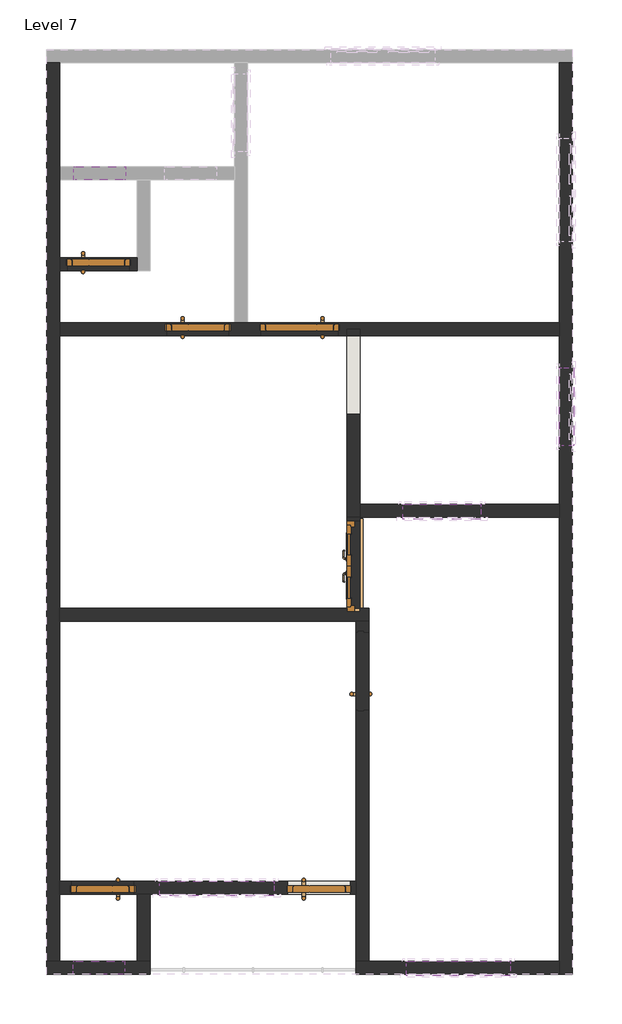
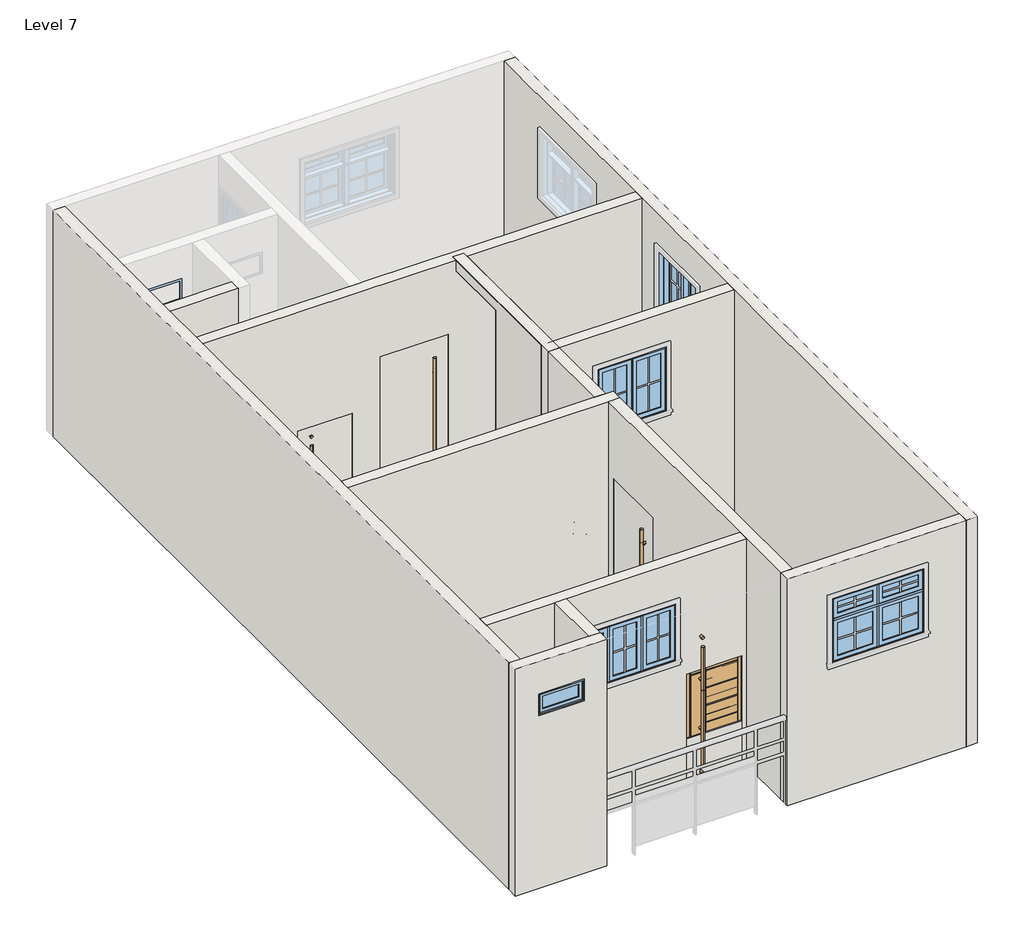
# One storey, part 1 of 2: 22 walls, 8 doors, 8 windows.
"""IFC4 building model written with IfcOpenShell, lengths in millimetres."""

from ifc_helpers import new_model, si_unit, frame, origin, place, context, project, spatial, polyline, outline, extrude, faceted_brep, transform, mapped, element, save
from components import door_9b787682, door_dc81b0c5, door_3_5c4206ef, door_3_79df91aa, door_2576ec39, door_55c03dfd, fixed_2_65c13adb, window_61697a4f, m_window_casement_double_3_e0bd8fa3, m_window_casement_double_awning_double_4_7efa9bbd

model = new_model("IFC4")

# Units and contexts
model_context = context("Model", 3, world=origin())
ifc_project = project(units=[si_unit("LENGTHUNIT", "METRE", prefix="MILLI")], contexts=[model_context])

# Site, building, storey
site = spatial("IfcSite", under=ifc_project)
building = spatial("IfcBuilding", under=site)
storey = spatial("IfcBuildingStorey", under=building, Name="Level 7", Elevation=10210.8)

# Doors
placement = place(None, origin())
door_shape = door_9b787682(model_context)
element("IfcDoor", 1, ObjectType="2'5\"", at=placement, inside=storey, context=model_context, shape_type="MappedRepresentation", body=[
    mapped(door_shape, transform((-22033.2963079, 3049.4742053, 10210.8), x_axis=(1.0, 0.0, 0.0), y_axis=(0.0, 1.0, 0.0), z_axis=(0.0, 0.0, 1.0))),
])
element("IfcDoor", 2, ObjectType="2'5\"", at=placement, inside=storey, context=model_context, shape_type="MappedRepresentation", body=[
    mapped(door_shape, transform((-23201.6963079, 3811.4742053, 10210.8), x_axis=(1.0, 0.0, 0.0), y_axis=(0.0, 1.0, 0.0), z_axis=(0.0, 0.0, 1.0))),
])
element("IfcDoor", 3, ObjectType="2'5\"", at=placement, inside=storey, context=model_context, shape_type="MappedRepresentation", body=[
    mapped(door_shape, transform((-23150.8963079, -3503.7257947, 10210.8), x_axis=(-1.0, 0.0, 0.0), y_axis=(0.0, -1.0, 0.0), z_axis=(0.0, 0.0, 1.0))),
])
door_2_shape = door_dc81b0c5(model_context)
element("IfcDoor", 4, ObjectType="2'5\"", at=placement, inside=storey, context=model_context, shape_type="MappedRepresentation", body=[
    mapped(door_2_shape, transform((-20610.8963079, -3503.7257947, 10257.0445349), x_axis=(1.0, 0.0, 0.0), y_axis=(0.0, 1.0, 0.0), z_axis=(0.0, 0.0, 1.0))),
])
element("IfcDoor", 5, ObjectType="2'5\"", at=placement, inside=storey, context=model_context, shape_type="MappedRepresentation", body=[
    mapped(door_2_shape, transform((-20610.8963079, -3503.7257947, 10866.6445349), x_axis=(1.0, 0.0, 0.0), y_axis=(0.0, 1.0, 0.0), z_axis=(0.0, 0.0, 1.0))),
])
door_3_shape = door_3_5c4206ef(model_context)
element("IfcDoor", 6, ObjectType="3'", at=placement, inside=storey, context=model_context, shape_type="MappedRepresentation", body=[
    mapped(door_3_shape, transform((-20102.8963079, -963.7257947, 10210.8), x_axis=(0.0, 1.0, 0.0), y_axis=(-1.0, 0.0, 0.0), z_axis=(0.0, 0.0, 1.0))),
])
door_3_2_shape = door_3_79df91aa(model_context)
element("IfcDoor", 7, ObjectType="3'", at=placement, inside=storey, context=model_context, shape_type="MappedRepresentation", body=[
    mapped(door_3_2_shape, transform((-20839.4963079, 3049.4742053, 10210.8), x_axis=(-1.0, 0.0, 0.0), y_axis=(0.0, -1.0, 0.0), z_axis=(0.0, 0.0, 1.0))),
])
door_4_shape = door_2576ec39(model_context)
door_5_shape = door_55c03dfd(model_context)
element("IfcDoor", 8, ObjectType="ExtDbl (8) : 3'6\"", at=placement, inside=storey, context=model_context, shape_type="MappedRepresentation", body=[
    mapped(door_4_shape, transform((-20204.4963079, 268.1742053, 10210.8), x_axis=(0.0, -1.0, 0.0), y_axis=(1.0, 0.0, 0.0), z_axis=(0.0, 0.0, 1.0))),
    mapped(door_5_shape, transform((-20204.4963079, 268.1742053, 10210.8), x_axis=(0.0, -1.0, 0.0), y_axis=(1.0, 0.0, 0.0), z_axis=(0.0, 0.0, 1.0))),
])

# Walls
element("IfcWall", 9, ObjectType="Generic - 6\"", at=placement, inside=storey, context=model_context, shape_type="Brep", body=[
    faceted_brep([(-17791.4963079, 6173.6742053, 10210.8), (-17791.4963079, 3125.6742053, 10210.8), (-17791.4963079, 2973.2742053, 10210.8), (-17791.4963079, 992.0742053, 10210.8), (-17791.4963079, 839.6742053, 10210.8), (-17791.4963079, -4367.3257947, 10210.8), (-17791.4963079, -4519.7257947, 10210.8), (-17791.4963079, -4519.7257947, 13411.2), (-17791.4963079, -4367.3257947, 13411.2), (-17791.4963079, 839.6742053, 13411.2), (-17791.4963079, 992.0742053, 13411.2), (-17791.4963079, 2973.2742053, 13411.2), (-17791.4963079, 3125.6742053, 13411.2), (-17791.4963079, 6173.6742053, 13411.2), (-17791.4963079, 4071.8242053, 12939.6), (-17791.4963079, 4071.8242053, 12039.6), (-17791.4963079, 5291.0242053, 12039.6), (-17791.4963079, 5291.0242053, 12939.6), (-17791.4963079, 1682.6367053, 12939.6), (-17791.4963079, 1682.6367053, 12039.6), (-17791.4963079, 2597.0367053, 12039.6), (-17791.4963079, 2597.0367053, 12939.6), (-17639.0963079, 6173.6742053, 10210.8), (-17639.0963079, 6173.6742053, 13411.2), (-17639.0963079, -4519.7257947, 13411.2), (-17639.0963079, -4519.7257947, 10210.8), (-17639.0963079, 4071.8242053, 12939.6), (-17639.0963079, 5291.0242053, 12939.6), (-17639.0963079, 5291.0242053, 12039.6), (-17639.0963079, 4071.8242053, 12039.6), (-17639.0963079, 1682.6367053, 12939.6), (-17639.0963079, 2597.0367053, 12939.6), (-17639.0963079, 2597.0367053, 12039.6), (-17639.0963079, 1682.6367053, 12039.6)], [[[0, 1, 2, 3, 4, 5, 6, 7, 8, 9, 10, 11, 12, 13], [14, 15, 16, 17], [18, 19, 20, 21]], [[22, 23, 24, 25], [26, 27, 28, 29], [30, 31, 32, 33]], [[6, 5, 4, 3, 2, 1, 0, 22, 25]], [[13, 12, 11, 10, 9, 8, 7, 24, 23]], [[0, 13, 23, 22]], [[7, 6, 25, 24]], [[15, 14, 26, 29]], [[16, 15, 29, 28]], [[17, 16, 28, 27]], [[14, 17, 27, 26]], [[19, 18, 30, 33]], [[20, 19, 33, 32]], [[21, 20, 32, 31]], [[18, 21, 31, 30]]]),
])
element("IfcWall", 10, ObjectType="Generic - 6\"", at=placement, inside=storey, context=model_context, shape_type="Brep", body=[
    faceted_brep([(-17791.4963079, -4367.3257947, 10210.8), (-20026.6963079, -4367.3257947, 10210.8), (-20179.0963079, -4367.3257947, 10210.8), (-20179.0963079, -4367.3257947, 13411.2), (-20026.6963079, -4367.3257947, 13411.2), (-17791.4963079, -4367.3257947, 13411.2), (-19585.5697454, -4367.3257947, 12939.6), (-19585.5697454, -4367.3257947, 12039.6), (-18366.3697454, -4367.3257947, 12039.6), (-18366.3697454, -4367.3257947, 12939.6), (-17791.4963079, -4519.7257947, 10210.8), (-17791.4963079, -4519.7257947, 13411.2), (-20179.0963079, -4519.7257947, 13411.2), (-20179.0963079, -4519.7257947, 10210.8), (-19585.5697454, -4519.7257947, 12939.6), (-18366.3697454, -4519.7257947, 12939.6), (-18366.3697454, -4519.7257947, 12039.6), (-19585.5697454, -4519.7257947, 12039.6)], [[[0, 1, 2, 3, 4, 5], [6, 7, 8, 9]], [[10, 11, 12, 13], [14, 15, 16, 17]], [[2, 1, 0, 10, 13]], [[5, 4, 3, 12, 11]], [[0, 5, 11, 10]], [[3, 2, 13, 12]], [[7, 6, 14, 17]], [[8, 7, 17, 16]], [[9, 8, 16, 15]], [[6, 9, 15, 14]]]),
])
element("IfcWall", 11, ObjectType="Generic - 6\"", at=placement, inside=storey, context=model_context, shape_type="Brep", body=[
    faceted_brep([(-23811.2963079, -4519.7257947, 10210.8), (-22592.0963079, -4519.7257947, 10210.8), (-22592.0963079, -4519.7257947, 13411.2), (-23811.2963079, -4519.7257947, 13411.2), (-23500.5431829, -4519.7257947, 12954.0), (-22890.9431829, -4519.7257947, 12954.0), (-22890.9431829, -4519.7257947, 12649.2), (-23500.5431829, -4519.7257947, 12649.2), (-23811.2963079, -4367.3257947, 10210.8), (-23811.2963079, -4367.3257947, 13411.2), (-23658.8963079, -4367.3257947, 13411.2), (-22744.4963079, -4367.3257947, 13411.2), (-22592.0963079, -4367.3257947, 13411.2), (-22592.0963079, -4367.3257947, 10210.8), (-22744.4963079, -4367.3257947, 10210.8), (-23658.8963079, -4367.3257947, 10210.8), (-23500.5431829, -4367.3257947, 12954.0), (-23500.5431829, -4367.3257947, 12649.2), (-22890.9431829, -4367.3257947, 12649.2), (-22890.9431829, -4367.3257947, 12954.0)], [[[0, 1, 2, 3], [4, 5, 6, 7]], [[8, 9, 10, 11, 12, 13, 14, 15], [16, 17, 18, 19]], [[1, 0, 8, 15, 14, 13]], [[3, 2, 12, 11, 10, 9]], [[0, 3, 9, 8]], [[2, 1, 13, 12]], [[17, 16, 4, 7]], [[18, 17, 7, 6]], [[19, 18, 6, 5]], [[16, 19, 5, 4]]]),
])
element("IfcWall", 12, ObjectType="Generic - 6\"", at=placement, inside=storey, context=model_context, shape_type="Brep", body=[
    faceted_brep([(-23658.8963079, -4367.3257947, 10210.8), (-23658.8963079, -3579.9257947, 10210.8), (-23658.8963079, -3427.5257947, 10210.8), (-23658.8963079, -379.5257947, 10210.8), (-23658.8963079, -227.1257947, 10210.8), (-23658.8963079, 2973.2742053, 10210.8), (-23658.8963079, 3125.6742053, 10210.8), (-23658.8963079, 3735.2742053, 10210.8), (-23658.8963079, 3887.6742053, 10210.8), (-23658.8963079, 4802.0742053, 10210.8), (-23658.8963079, 4954.4742053, 10210.8), (-23658.8963079, 6173.6742053, 10210.8), (-23658.8963079, 6173.6742053, 13411.2), (-23658.8963079, 4954.4742053, 13411.2), (-23658.8963079, 4802.0742053, 13411.2), (-23658.8963079, 3887.6742053, 13411.2), (-23658.8963079, 3735.2742053, 13411.2), (-23658.8963079, 3125.6742053, 13411.2), (-23658.8963079, 2973.2742053, 13411.2), (-23658.8963079, -227.1257947, 13411.2), (-23658.8963079, -379.5257947, 13411.2), (-23658.8963079, -3427.5257947, 13411.2), (-23658.8963079, -3579.9257947, 13411.2), (-23658.8963079, -4367.3257947, 13411.2), (-23811.2963079, -4367.3257947, 10210.8), (-23811.2963079, -4367.3257947, 13411.2), (-23811.2963079, 6173.6742053, 13411.2), (-23811.2963079, 6173.6742053, 10210.8)], [[[0, 1, 2, 3, 4, 5, 6, 7, 8, 9, 10, 11, 12, 13, 14, 15, 16, 17, 18, 19, 20, 21, 22, 23]], [[24, 25, 26, 27]], [[11, 10, 9, 8, 7, 6, 5, 4, 3, 2, 1, 0, 24, 27]], [[23, 22, 21, 20, 19, 18, 17, 16, 15, 14, 13, 12, 26, 25]], [[12, 11, 27, 26]], [[0, 23, 25, 24]]]),
])
element("IfcWall", 13, ObjectType="Generic - 6\"", at=placement, inside=storey, context=model_context, shape_type="Brep", body=[
    faceted_brep([(-17791.4963079, 2973.2742053, 13411.2), (-20128.2963079, 2973.2742053, 13411.2), (-20280.6963079, 2973.2742053, 13411.2), (-23658.8963079, 2973.2742053, 13411.2), (-23658.8963079, 2973.2742053, 10210.8), (-22401.5963079, 2973.2742053, 10210.8), (-22401.5963079, 2973.2742053, 11734.8), (-21664.9963079, 2973.2742053, 11734.8), (-21664.9963079, 2973.2742053, 10210.8), (-21296.6963079, 2973.2742053, 10210.8), (-21296.6963079, 2973.2742053, 12400.3), (-20382.2963079, 2973.2742053, 12400.3), (-20382.2963079, 2973.2742053, 10210.8), (-20280.6963079, 2973.2742053, 10210.8), (-20128.2963079, 2973.2742053, 10210.8), (-17791.4963079, 2973.2742053, 10210.8), (-23658.8963079, 3125.6742053, 13411.2), (-21601.4963079, 3125.6742053, 13411.2), (-21449.0963079, 3125.6742053, 13411.2), (-17791.4963079, 3125.6742053, 13411.2), (-17791.4963079, 3125.6742053, 10210.8), (-20382.2963079, 3125.6742053, 10210.8), (-20382.2963079, 3125.6742053, 12400.3), (-21296.6963079, 3125.6742053, 12400.3), (-21296.6963079, 3125.6742053, 10210.8), (-21449.0963079, 3125.6742053, 10210.8), (-21601.4963079, 3125.6742053, 10210.8), (-21664.9963079, 3125.6742053, 10210.8), (-21664.9963079, 3125.6742053, 11734.8), (-22401.5963079, 3125.6742053, 11734.8), (-22401.5963079, 3125.6742053, 10210.8), (-23658.8963079, 3125.6742053, 10210.8), (-22401.5963079, 3105.6742053, 10210.8), (-22416.5963079, 3105.6742053, 10210.8), (-22416.5963079, 3028.6742053, 10210.8), (-22401.5963079, 3028.6742053, 10210.8), (-20382.2963079, 3028.6742053, 10210.8), (-20367.2963079, 3028.6742053, 10210.8), (-20367.2963079, 3105.6742053, 10210.8), (-20382.2963079, 3105.6742053, 10210.8), (-21296.6963079, 3028.6742053, 10210.8), (-21664.9963079, 3028.6742053, 10210.8), (-21649.9963079, 3028.6742053, 10210.8), (-21649.9963079, 3105.6742053, 10210.8), (-21664.9963079, 3105.6742053, 10210.8), (-21296.6963079, 3105.6742053, 10210.8), (-21311.6963079, 3105.6742053, 10210.8), (-21311.6963079, 3028.6742053, 10210.8), (-21296.6963079, 3105.6742053, 12400.3), (-20382.2963079, 3105.6742053, 12400.3), (-20382.2963079, 3028.6742053, 12400.3), (-21296.6963079, 3028.6742053, 12400.3), (-21311.6963079, 3105.6742053, 12415.3), (-20367.2963079, 3105.6742053, 12415.3), (-20367.2963079, 3028.6742053, 12415.3), (-21311.6963079, 3028.6742053, 12415.3), (-21664.9963079, 3105.6742053, 11734.8), (-22401.5963079, 3105.6742053, 11734.8), (-22401.5963079, 3028.6742053, 11734.8), (-21664.9963079, 3028.6742053, 11734.8), (-22416.5963079, 3105.6742053, 11749.8), (-21649.9963079, 3105.6742053, 11749.8), (-21649.9963079, 3028.6742053, 11749.8), (-22416.5963079, 3028.6742053, 11749.8)], [[[0, 1, 2, 3, 4, 5, 6, 7, 8, 9, 10, 11, 12, 13, 14, 15]], [[16, 17, 18, 19, 20, 21, 22, 23, 24, 25, 26, 27, 28, 29, 30, 31]], [[4, 31, 30, 32, 33, 34, 35, 5]], [[20, 15, 14, 13, 12, 36, 37, 38, 39, 21]], [[40, 9, 8, 41, 42, 43, 44, 27, 26, 25, 24, 45, 46, 47]], [[3, 2, 1, 0, 19, 18, 17, 16]], [[0, 15, 20, 19]], [[4, 3, 16, 31]], [[48, 23, 22, 49]], [[50, 11, 10, 51]], [[23, 48, 45, 24]], [[51, 10, 9, 40]], [[49, 22, 21, 39]], [[11, 50, 36, 12]], [[52, 53, 54, 55]], [[52, 55, 47, 46]], [[50, 51, 40, 47, 55, 54, 37, 36]], [[54, 53, 38, 37]], [[48, 49, 39, 38, 53, 52, 46, 45]], [[28, 56, 57, 29]], [[6, 58, 59, 7]], [[56, 28, 27, 44]], [[7, 59, 41, 8]], [[29, 57, 32, 30]], [[58, 6, 5, 35]], [[60, 61, 62, 63]], [[62, 61, 43, 42]], [[59, 58, 35, 34, 63, 62, 42, 41]], [[60, 63, 34, 33]], [[57, 56, 44, 43, 61, 60, 33, 32]]]),
])
element("IfcWall", 14, ObjectType="Generic - 6\"", at=placement, inside=storey, context=model_context, shape_type="Brep", body=[
    faceted_brep([(-20280.6963079, 3049.4742053, 13411.2), (-20280.6963079, 3049.4742053, 10210.8), (-20280.6963079, 839.6742053, 10210.8), (-20280.6963079, 839.6742053, 13411.2), (-20280.6963079, 2974.7724011, 13258.8), (-20280.6963079, 2050.5574639, 13258.8), (-20280.6963079, 2050.5574639, 10820.4), (-20280.6963079, 2974.7724011, 10820.4), (-20128.2963079, 839.6742053, 10210.8), (-20128.2963079, 992.0742053, 10210.8), (-20128.2963079, 3049.4742053, 10210.8), (-20128.2963079, 3049.4742053, 13411.2), (-20128.2963079, 992.0742053, 13411.2), (-20128.2963079, 839.6742053, 13411.2), (-20128.2963079, 2050.5574639, 13258.8), (-20128.2963079, 2974.7724011, 13258.8), (-20128.2963079, 2974.7724011, 10820.4), (-20128.2963079, 2050.5574639, 10820.4)], [[[0, 1, 2, 3], [4, 5, 6, 7]], [[8, 9, 10, 11, 12, 13], [14, 15, 16, 17]], [[2, 1, 10, 9, 8]], [[0, 3, 13, 12, 11]], [[3, 2, 8, 13]], [[4, 15, 14, 5]], [[6, 17, 16, 7]], [[15, 4, 7, 16]], [[5, 14, 17, 6]], [[0, 11, 10, 1]]]),
])
element("IfcWall", 15, ObjectType="Generic - 6\"", at=placement, inside=storey, context=model_context, shape_type="SweptSolid", body=[
    extrude(outline(polyline([(10210.8, -20128.2963079), (10210.8, -17791.4963079), (13411.2, -17791.4963079), (13411.2, -20128.2963079), (10210.8, -20128.2963079)]), holes=[polyline([(12939.6, -19624.1658391), (12939.6, -18709.7658391), (12039.6, -18709.7658391), (12039.6, -19624.1658391), (12939.6, -19624.1658391)])]), frame((0.0, 839.6742053, 0.0), z_axis=(0.0, 1.0, 0.0), x_axis=(0.0, 0.0, 1.0)), (0.0, 0.0, 1.0), 152.4),
])
element("IfcWall", 16, ObjectType="Generic - 6\"", at=placement, inside=storey, context=model_context, shape_type="Brep", body=[
    faceted_brep([(-23658.8963079, -379.5257947, 10210.8), (-20179.0963079, -379.5257947, 10210.8), (-20026.6963079, -379.5257947, 10210.8), (-20026.6963079, -379.5257947, 13411.2), (-20179.0963079, -379.5257947, 13411.2), (-23658.8963079, -379.5257947, 13411.2), (-23658.8963079, -227.1257947, 13411.2), (-20280.6963079, -227.1257947, 13411.2), (-20128.2963079, -227.1257947, 13411.2), (-20026.6963079, -227.1257947, 13411.2), (-20026.6963079, -227.1257947, 10210.8), (-20128.2963079, -227.1257947, 10210.8), (-20128.2963079, -227.1257947, 12320.8), (-20280.6963079, -227.1257947, 12320.8), (-20280.6963079, -227.1257947, 10210.8), (-23658.8963079, -227.1257947, 10210.8), (-20280.6963079, -265.2257947, 10210.8), (-20128.2963079, -265.2257947, 10210.8), (-20280.6963079, -265.2257947, 12320.8), (-20128.2963079, -265.2257947, 12320.8)], [[[0, 1, 2, 3, 4, 5]], [[6, 7, 8, 9, 10, 11, 12, 13, 14, 15]], [[2, 1, 0, 15, 14, 16, 17, 11, 10]], [[5, 4, 3, 9, 8, 7, 6]], [[0, 5, 6, 15]], [[3, 2, 10, 9]], [[18, 16, 14, 13]], [[17, 19, 12, 11]], [[19, 18, 13, 12]], [[16, 18, 19, 17]]]),
])
element("IfcWall", 17, ObjectType="Generic - 6\"", at=placement, inside=storey, context=model_context, shape_type="Brep", body=[
    faceted_brep([(-20179.0963079, -4367.3257947, 13411.2), (-20179.0963079, -3579.9257947, 13411.2), (-20179.0963079, -3427.5257947, 13411.2), (-20179.0963079, -379.5257947, 13411.2), (-20179.0963079, -379.5257947, 10210.8), (-20179.0963079, -506.5257947, 10210.8), (-20179.0963079, -506.5257947, 12400.3), (-20179.0963079, -1420.9257947, 12400.3), (-20179.0963079, -1420.9257947, 10210.8), (-20179.0963079, -3427.5257947, 10210.8), (-20179.0963079, -3579.9257947, 10210.8), (-20179.0963079, -4367.3257947, 10210.8), (-20026.6963079, -379.5257947, 13411.2), (-20026.6963079, -4367.3257947, 13411.2), (-20026.6963079, -4367.3257947, 10210.8), (-20026.6963079, -1420.9257947, 10210.8), (-20026.6963079, -1420.9257947, 12400.3), (-20026.6963079, -506.5257947, 12400.3), (-20026.6963079, -506.5257947, 10210.8), (-20026.6963079, -379.5257947, 10210.8), (-20082.0963079, -506.5257947, 10210.8), (-20082.0963079, -491.5257947, 10210.8), (-20159.0963079, -491.5257947, 10210.8), (-20159.0963079, -506.5257947, 10210.8), (-20159.0963079, -1420.9257947, 10210.8), (-20159.0963079, -1435.9257947, 10210.8), (-20082.0963079, -1435.9257947, 10210.8), (-20082.0963079, -1420.9257947, 10210.8), (-20159.0963079, -506.5257947, 12400.3), (-20159.0963079, -1420.9257947, 12400.3), (-20082.0963079, -1420.9257947, 12400.3), (-20082.0963079, -506.5257947, 12400.3), (-20159.0963079, -1435.9257947, 12415.3), (-20159.0963079, -491.5257947, 12415.3), (-20082.0963079, -491.5257947, 12415.3), (-20082.0963079, -1435.9257947, 12415.3)], [[[0, 1, 2, 3, 4, 5, 6, 7, 8, 9, 10, 11]], [[12, 13, 14, 15, 16, 17, 18, 19]], [[4, 19, 18, 20, 21, 22, 23, 5]], [[14, 11, 10, 9, 8, 24, 25, 26, 27, 15]], [[3, 2, 1, 0, 13, 12]], [[0, 11, 14, 13]], [[4, 3, 12, 19]], [[6, 28, 29, 7]], [[16, 30, 31, 17]], [[28, 6, 5, 23]], [[17, 31, 20, 18]], [[7, 29, 24, 8]], [[30, 16, 15, 27]], [[32, 33, 34, 35]], [[34, 33, 22, 21]], [[31, 30, 27, 26, 35, 34, 21, 20]], [[32, 35, 26, 25]], [[29, 28, 23, 22, 33, 32, 25, 24]]]),
])
element("IfcWall", 18, ObjectType="Generic - 6\"", at=placement, inside=storey, context=model_context, shape_type="Brep", body=[
    faceted_brep([(-20179.0963079, -3579.9257947, 13411.2), (-22592.0963079, -3579.9257947, 13411.2), (-22744.4963079, -3579.9257947, 13411.2), (-23658.8963079, -3579.9257947, 13411.2), (-23658.8963079, -3579.9257947, 10210.8), (-23519.1963079, -3579.9257947, 10210.8), (-23519.1963079, -3579.9257947, 11734.8), (-22782.5963079, -3579.9257947, 11734.8), (-22782.5963079, -3579.9257947, 10210.8), (-22744.4963079, -3579.9257947, 10210.8), (-22592.0963079, -3579.9257947, 10210.8), (-20179.0963079, -3579.9257947, 10210.8), (-22484.1463079, -3579.9257947, 12039.6), (-22484.1463079, -3579.9257947, 12839.6), (-21137.9463079, -3579.9257947, 12839.6), (-21137.9463079, -3579.9257947, 12039.6), (-20979.1963079, -3579.9257947, 11781.0445349), (-20242.5963079, -3579.9257947, 11781.0445349), (-20242.5963079, -3579.9257947, 10257.0445349), (-20979.1963079, -3579.9257947, 10257.0445349), (-23658.8963079, -3427.5257947, 13411.2), (-20179.0963079, -3427.5257947, 13411.2), (-20179.0963079, -3427.5257947, 10210.8), (-22782.5963079, -3427.5257947, 10210.8), (-22782.5963079, -3427.5257947, 11734.8), (-23519.1963079, -3427.5257947, 11734.8), (-23519.1963079, -3427.5257947, 10210.8), (-23658.8963079, -3427.5257947, 10210.8), (-22484.1463079, -3427.5257947, 12839.6), (-22484.1463079, -3427.5257947, 12039.6), (-21137.9463079, -3427.5257947, 12039.6), (-21137.9463079, -3427.5257947, 12839.6), (-20242.5963079, -3427.5257947, 11781.0445349), (-20979.1963079, -3427.5257947, 11781.0445349), (-20979.1963079, -3427.5257947, 10257.0445349), (-20242.5963079, -3427.5257947, 10257.0445349), (-23519.1963079, -3482.9257947, 10210.8), (-23534.1963079, -3482.9257947, 10210.8), (-23534.1963079, -3559.9257947, 10210.8), (-23519.1963079, -3559.9257947, 10210.8), (-22782.5963079, -3559.9257947, 10210.8), (-22767.5963079, -3559.9257947, 10210.8), (-22767.5963079, -3482.9257947, 10210.8), (-22782.5963079, -3482.9257947, 10210.8), (-20979.1963079, -3559.9257947, 11781.0445349), (-20242.5963079, -3559.9257947, 11781.0445349), (-20242.5963079, -3482.9257947, 11781.0445349), (-20979.1963079, -3482.9257947, 11781.0445349), (-20242.5963079, -3559.9257947, 10257.0445349), (-20242.5963079, -3482.9257947, 10257.0445349), (-20227.5963079, -3559.9257947, 10257.0445349), (-20227.5963079, -3482.9257947, 10257.0445349), (-20979.1963079, -3482.9257947, 10257.0445349), (-20994.1963079, -3482.9257947, 10257.0445349), (-20994.1963079, -3559.9257947, 10257.0445349), (-20979.1963079, -3559.9257947, 10257.0445349), (-20994.1963079, -3559.9257947, 11796.0445349), (-20994.1963079, -3482.9257947, 11796.0445349), (-20227.5963079, -3482.9257947, 11796.0445349), (-20227.5963079, -3559.9257947, 11796.0445349), (-23519.1963079, -3559.9257947, 11734.8), (-22782.5963079, -3559.9257947, 11734.8), (-22782.5963079, -3482.9257947, 11734.8), (-23519.1963079, -3482.9257947, 11734.8), (-22767.5963079, -3559.9257947, 11749.8), (-23534.1963079, -3559.9257947, 11749.8), (-23534.1963079, -3482.9257947, 11749.8), (-22767.5963079, -3482.9257947, 11749.8)], [[[0, 1, 2, 3, 4, 5, 6, 7, 8, 9, 10, 11], [12, 13, 14, 15], [16, 17, 18, 19]], [[20, 21, 22, 23, 24, 25, 26, 27], [28, 29, 30, 31], [32, 33, 34, 35]], [[4, 27, 26, 36, 37, 38, 39, 5]], [[22, 11, 10, 9, 8, 40, 41, 42, 43, 23]], [[3, 2, 1, 0, 21, 20]], [[4, 3, 20, 27]], [[0, 11, 22, 21]], [[29, 28, 13, 12]], [[30, 29, 12, 15]], [[31, 30, 15, 14]], [[28, 31, 14, 13]], [[16, 44, 45, 17]], [[32, 46, 47, 33]], [[17, 45, 48, 18]], [[46, 32, 35, 49]], [[18, 48, 50, 51, 49, 35, 34, 52, 53, 54, 55, 19]], [[44, 16, 19, 55]], [[33, 47, 52, 34]], [[56, 57, 58, 59]], [[51, 50, 59, 58]], [[47, 46, 49, 51, 58, 57, 53, 52]], [[54, 53, 57, 56]], [[45, 44, 55, 54, 56, 59, 50, 48]], [[6, 60, 61, 7]], [[24, 62, 63, 25]], [[60, 6, 5, 39]], [[25, 63, 36, 26]], [[7, 61, 40, 8]], [[62, 24, 23, 43]], [[64, 65, 66, 67]], [[66, 65, 38, 37]], [[63, 62, 43, 42, 67, 66, 37, 36]], [[64, 67, 42, 41]], [[61, 60, 39, 38, 65, 64, 41, 40]]]),
])
element("IfcWall", 19, ObjectType="Generic - 6\"", at=placement, inside=storey, context=model_context, shape_type="SweptSolid", body=[
    extrude(outline(polyline([(-22744.4963079, -4367.3257947), (-22744.4963079, -3579.9257947), (-22592.0963079, -3579.9257947), (-22592.0963079, -4367.3257947), (-22744.4963079, -4367.3257947)])), frame((0.0, 0.0, 10210.8), z_axis=(0.0, 0.0, 1.0), x_axis=(1.0, 0.0, 0.0)), (0.0, 0.0, 1.0), 3200.4),
])
element("IfcWall", 20, ObjectType="Generic - 6\"", at=placement, inside=storey, context=model_context, shape_type="Brep", body=[
    faceted_brep([(-22744.4963079, 3735.2742053, 13411.2), (-23658.8963079, 3735.2742053, 13411.2), (-23658.8963079, 3735.2742053, 10210.8), (-23569.9963079, 3735.2742053, 10210.8), (-23569.9963079, 3735.2742053, 11734.8), (-22833.3963079, 3735.2742053, 11734.8), (-22833.3963079, 3735.2742053, 10210.8), (-22744.4963079, 3735.2742053, 10210.8), (-23658.8963079, 3887.6742053, 13411.2), (-22744.4963079, 3887.6742053, 13411.2), (-22744.4963079, 3887.6742053, 10210.8), (-22833.3963079, 3887.6742053, 10210.8), (-22833.3963079, 3887.6742053, 11734.8), (-23569.9963079, 3887.6742053, 11734.8), (-23569.9963079, 3887.6742053, 10210.8), (-23658.8963079, 3887.6742053, 10210.8), (-23569.9963079, 3867.6742053, 10210.8), (-23584.9963079, 3867.6742053, 10210.8), (-23584.9963079, 3790.6742053, 10210.8), (-23569.9963079, 3790.6742053, 10210.8), (-22833.3963079, 3790.6742053, 10210.8), (-22818.3963079, 3790.6742053, 10210.8), (-22818.3963079, 3867.6742053, 10210.8), (-22833.3963079, 3867.6742053, 10210.8), (-22833.3963079, 3867.6742053, 11734.8), (-23569.9963079, 3867.6742053, 11734.8), (-23569.9963079, 3790.6742053, 11734.8), (-22833.3963079, 3790.6742053, 11734.8), (-23584.9963079, 3867.6742053, 11749.8), (-22818.3963079, 3867.6742053, 11749.8), (-22818.3963079, 3790.6742053, 11749.8), (-23584.9963079, 3790.6742053, 11749.8)], [[[0, 1, 2, 3, 4, 5, 6, 7]], [[8, 9, 10, 11, 12, 13, 14, 15]], [[2, 15, 14, 16, 17, 18, 19, 3]], [[10, 7, 6, 20, 21, 22, 23, 11]], [[1, 0, 9, 8]], [[0, 7, 10, 9]], [[2, 1, 8, 15]], [[12, 24, 25, 13]], [[4, 26, 27, 5]], [[24, 12, 11, 23]], [[5, 27, 20, 6]], [[13, 25, 16, 14]], [[26, 4, 3, 19]], [[28, 29, 30, 31]], [[30, 29, 22, 21]], [[27, 26, 19, 18, 31, 30, 21, 20]], [[28, 31, 18, 17]], [[25, 24, 23, 22, 29, 28, 17, 16]]]),
])
element("IfcWall", 21, ObjectType="Generic - 6\"", at=placement, inside=storey, context=model_context, shape_type="Brep", body=[
    faceted_brep([(-20280.6963079, -227.1257947, 13411.2), (-20280.6963079, 839.6742053, 13411.2), (-20280.6963079, 839.6742053, 10210.8), (-20280.6963079, 801.5742053, 10210.8), (-20280.6963079, 801.5742053, 12320.8), (-20280.6963079, -227.1257947, 12320.8), (-20128.2963079, 839.6742053, 13411.2), (-20128.2963079, -227.1257947, 13411.2), (-20128.2963079, -227.1257947, 12320.8), (-20128.2963079, 801.5742053, 12320.8), (-20128.2963079, 801.5742053, 10210.8), (-20128.2963079, 839.6742053, 10210.8), (-20179.0963079, -227.1257947, 13411.2), (-20179.0963079, -227.1257947, 12320.8)], [[[0, 1, 2, 3, 4, 5]], [[6, 7, 8, 9, 10, 11]], [[2, 11, 10, 3]], [[1, 0, 12, 7, 6]], [[2, 1, 6, 11]], [[7, 12, 0, 5, 13, 8]], [[4, 9, 8, 13, 5]], [[9, 4, 3, 10]]]),
])
element("IfcWall", 22, ObjectType="Generic - 6\"", at=placement, inside=storey, context=model_context, shape_type="Brep", body=[
    faceted_brep([(-23658.8963079, 2973.2742053, 10210.8), (-20280.6963079, 2973.2742053, 10210.8), (-20128.2963079, 2973.2742053, 10210.8), (-17791.4963079, 2973.2742053, 10210.8), (-17791.4963079, 2973.2742053, 13411.2), (-20128.2963079, 2973.2742053, 13411.2), (-20280.6963079, 2973.2742053, 13411.2), (-23658.8963079, 2973.2742053, 13411.2), (-23658.8963079, 3125.6742053, 10210.8), (-23658.8963079, 3125.6742053, 13411.2), (-21601.4963079, 3125.6742053, 13411.2), (-21449.0963079, 3125.6742053, 13411.2), (-17791.4963079, 3125.6742053, 13411.2), (-17791.4963079, 3125.6742053, 10210.8), (-21449.0963079, 3125.6742053, 10210.8), (-21601.4963079, 3125.6742053, 10210.8)], [[[0, 1, 2, 3, 4, 5, 6, 7]], [[8, 9, 10, 11, 12, 13, 14, 15]], [[3, 2, 1, 0, 8, 15, 14, 13]], [[7, 6, 5, 4, 12, 11, 10, 9]], [[0, 7, 9, 8]], [[4, 3, 13, 12]]]),
])
element("IfcWall", 23, ObjectType="Generic - 6\"", at=placement, inside=storey, context=model_context, shape_type="SweptSolid", body=[
    extrude(outline(polyline([(2973.2742053, 10210.8), (992.0742053, 10210.8), (992.0742053, 13411.2), (2973.2742053, 13411.2), (2973.2742053, 13258.8), (2050.5574639, 13258.8), (2050.5574639, 10820.4), (2973.2742053, 10820.4), (2973.2742053, 10210.8)])), frame((-20280.6963079, 0.0, 0.0), z_axis=(1.0, 0.0, 0.0), x_axis=(0.0, 1.0, 0.0)), (0.0, 0.0, 1.0), 152.4),
])
element("IfcWall", 24, ObjectType="Generic - 6\"", at=placement, inside=storey, context=model_context, shape_type="SweptSolid", body=[
    extrude(outline(polyline([(10210.8, -20128.2963079), (10210.8, -17791.4963079), (13411.2, -17791.4963079), (13411.2, -20128.2963079), (10210.8, -20128.2963079)]), holes=[polyline([(12939.6, -19624.1658391), (12939.6, -18709.7658391), (12039.6, -18709.7658391), (12039.6, -19624.1658391), (12939.6, -19624.1658391)])]), frame((0.0, 839.6742053, 0.0), z_axis=(0.0, 1.0, 0.0), x_axis=(0.0, 0.0, 1.0)), (0.0, 0.0, 1.0), 152.4),
])
element("IfcWall", 25, ObjectType="Generic - 6\"", at=placement, inside=storey, context=model_context, shape_type="Brep", body=[
    faceted_brep([(-23658.8963079, -379.5257947, 10210.8), (-20179.0963079, -379.5257947, 10210.8), (-20179.0963079, -379.5257947, 13411.2), (-23658.8963079, -379.5257947, 13411.2), (-23658.8963079, -227.1257947, 13411.2), (-20280.6963079, -227.1257947, 13411.2), (-20179.0963079, -227.1257947, 13411.2), (-20179.0963079, -227.1257947, 12320.8), (-20280.6963079, -227.1257947, 12320.8), (-20280.6963079, -227.1257947, 10210.8), (-23658.8963079, -227.1257947, 10210.8), (-20280.6963079, -265.2257947, 10210.8), (-20179.0963079, -265.2257947, 10210.8), (-20179.0963079, -265.2257947, 12320.8), (-20280.6963079, -265.2257947, 12320.8)], [[[0, 1, 2, 3]], [[4, 5, 6, 7, 8, 9, 10]], [[1, 0, 10, 9, 11, 12]], [[3, 2, 6, 5, 4]], [[2, 1, 12, 13, 7, 6]], [[14, 11, 9, 8]], [[11, 14, 13, 12]], [[14, 8, 7, 13]], [[0, 3, 4, 10]]]),
])
element("IfcWall", 26, ObjectType="Generic - 6\"", at=placement, inside=storey, context=model_context, shape_type="Brep", body=[
    faceted_brep([(-20179.0963079, -379.5257947, 10210.8), (-20179.0963079, -3427.5257947, 10210.8), (-20179.0963079, -3579.9257947, 10210.8), (-20179.0963079, -4367.3257947, 10210.8), (-20179.0963079, -4367.3257947, 13411.2), (-20179.0963079, -3579.9257947, 13411.2), (-20179.0963079, -3427.5257947, 13411.2), (-20179.0963079, -379.5257947, 13411.2), (-20026.6963079, -379.5257947, 10210.8), (-20026.6963079, -379.5257947, 13411.2), (-20026.6963079, -4367.3257947, 13411.2), (-20026.6963079, -4367.3257947, 10210.8)], [[[0, 1, 2, 3, 4, 5, 6, 7]], [[8, 9, 10, 11]], [[3, 2, 1, 0, 8, 11]], [[7, 6, 5, 4, 10, 9]], [[4, 3, 11, 10]], [[0, 7, 9, 8]]]),
])
element("IfcWall", 27, ObjectType="Generic - 6\"", at=placement, inside=storey, context=model_context, shape_type="Brep", body=[
    faceted_brep([(-23658.8963079, -3579.9257947, 10210.8), (-22744.4963079, -3579.9257947, 10210.8), (-22592.0963079, -3579.9257947, 10210.8), (-20179.0963079, -3579.9257947, 10210.8), (-20179.0963079, -3579.9257947, 13411.2), (-22592.0963079, -3579.9257947, 13411.2), (-22744.4963079, -3579.9257947, 13411.2), (-23658.8963079, -3579.9257947, 13411.2), (-22484.1463079, -3579.9257947, 12039.6), (-22484.1463079, -3579.9257947, 12839.6), (-21137.9463079, -3579.9257947, 12839.6), (-21137.9463079, -3579.9257947, 12039.6), (-20979.1963079, -3579.9257947, 12390.6445349), (-20242.5963079, -3579.9257947, 12390.6445349), (-20242.5963079, -3579.9257947, 10866.6445349), (-20979.1963079, -3579.9257947, 10866.6445349), (-20179.0963079, -3427.5257947, 10210.8), (-23658.8963079, -3427.5257947, 10210.8), (-23658.8963079, -3427.5257947, 13411.2), (-20179.0963079, -3427.5257947, 13411.2), (-22484.1463079, -3427.5257947, 12839.6), (-22484.1463079, -3427.5257947, 12039.6), (-21137.9463079, -3427.5257947, 12039.6), (-21137.9463079, -3427.5257947, 12839.6), (-20242.5963079, -3427.5257947, 12390.6445349), (-20979.1963079, -3427.5257947, 12390.6445349), (-20979.1963079, -3427.5257947, 10866.6445349), (-20242.5963079, -3427.5257947, 10866.6445349), (-20979.1963079, -3559.9257947, 12390.6445349), (-20242.5963079, -3559.9257947, 12390.6445349), (-20242.5963079, -3482.9257947, 12390.6445349), (-20979.1963079, -3482.9257947, 12390.6445349), (-20242.5963079, -3559.9257947, 10866.6445349), (-20242.5963079, -3482.9257947, 10866.6445349), (-20227.5963079, -3559.9257947, 10866.6445349), (-20227.5963079, -3482.9257947, 10866.6445349), (-20979.1963079, -3482.9257947, 10866.6445349), (-20994.1963079, -3482.9257947, 10866.6445349), (-20994.1963079, -3559.9257947, 10866.6445349), (-20979.1963079, -3559.9257947, 10866.6445349), (-20994.1963079, -3559.9257947, 12405.6445349), (-20994.1963079, -3482.9257947, 12405.6445349), (-20227.5963079, -3482.9257947, 12405.6445349), (-20227.5963079, -3559.9257947, 12405.6445349)], [[[0, 1, 2, 3, 4, 5, 6, 7], [8, 9, 10, 11], [12, 13, 14, 15]], [[16, 17, 18, 19], [20, 21, 22, 23], [24, 25, 26, 27]], [[3, 2, 1, 0, 17, 16]], [[7, 6, 5, 4, 19, 18]], [[4, 3, 16, 19]], [[21, 20, 9, 8]], [[22, 21, 8, 11]], [[23, 22, 11, 10]], [[20, 23, 10, 9]], [[12, 28, 29, 13]], [[24, 30, 31, 25]], [[13, 29, 32, 14]], [[30, 24, 27, 33]], [[14, 32, 34, 35, 33, 27, 26, 36, 37, 38, 39, 15]], [[28, 12, 15, 39]], [[25, 31, 36, 26]], [[40, 41, 42, 43]], [[35, 34, 43, 42]], [[31, 30, 33, 35, 42, 41, 37, 36]], [[38, 37, 41, 40]], [[29, 28, 39, 38, 40, 43, 34, 32]], [[0, 7, 18, 17]]]),
])
element("IfcWall", 28, ObjectType="Generic - 6\"", at=placement, inside=storey, context=model_context, shape_type="SweptSolid", body=[
    extrude(outline(polyline([(-22744.4963079, -4367.3257947), (-22744.4963079, -3579.9257947), (-22592.0963079, -3579.9257947), (-22592.0963079, -4367.3257947), (-22744.4963079, -4367.3257947)])), frame((0.0, 0.0, 10210.8), z_axis=(0.0, 0.0, 1.0), x_axis=(1.0, 0.0, 0.0)), (0.0, 0.0, 1.0), 3200.4),
])
element("IfcWall", 29, ObjectType="Generic - 6\"", at=placement, inside=storey, context=model_context, shape_type="SweptSolid", body=[
    extrude(outline(polyline([(-22744.4963079, 3735.2742053), (-23658.8963079, 3735.2742053), (-23658.8963079, 3887.6742053), (-22744.4963079, 3887.6742053), (-22744.4963079, 3735.2742053)])), frame((0.0, 0.0, 10210.8), z_axis=(0.0, 0.0, 1.0), x_axis=(1.0, 0.0, 0.0)), (0.0, 0.0, 1.0), 3200.4),
])
element("IfcWall", 30, ObjectType="Generic - 6\"", at=placement, inside=storey, context=model_context, shape_type="Brep", body=[
    faceted_brep([(-20280.6963079, 839.6742053, 10210.8), (-20280.6963079, -227.1257947, 10210.8), (-20280.6963079, -227.1257947, 13411.2), (-20280.6963079, 839.6742053, 13411.2), (-20128.2963079, 839.6742053, 10210.8), (-20128.2963079, 839.6742053, 13411.2), (-20128.2963079, -227.1257947, 13411.2), (-20128.2963079, -227.1257947, 10210.8), (-20179.0963079, -227.1257947, 13411.2)], [[[0, 1, 2, 3]], [[4, 5, 6, 7]], [[1, 0, 4, 7]], [[3, 2, 8, 6, 5]], [[2, 1, 7, 6, 8]], [[0, 3, 5, 4]]]),
])

# Windows
fixed_2_shape = fixed_2_65c13adb(model_context)
element("IfcWindow", 31, ObjectType="Fixed : 2'", at=placement, inside=storey, context=model_context, shape_type="MappedRepresentation", body=[
    mapped(fixed_2_shape, transform((-23233.8431829, -4443.5257947, 11734.8), x_axis=(-1.0, 0.0, 0.0), y_axis=(0.0, -1.0, 0.0), z_axis=(0.0, 0.0, 1.0))),
])
element("IfcWindow", 32, ObjectType="Fixed : 2'", at=placement, inside=storey, context=model_context, shape_type="MappedRepresentation", body=[
    mapped(fixed_2_shape, transform((-23147.2252141, 4878.2742053, 11734.8), x_axis=(1.0, 0.0, 0.0), y_axis=(0.0, 1.0, 0.0), z_axis=(0.0, 0.0, 1.0))),
])
window_shape = window_61697a4f(model_context)
element("IfcWindow", 33, ObjectType="M_Window-Awning-Triple-Horizontal : 4'5\"", at=placement, inside=storey, context=model_context, shape_type="MappedRepresentation", body=[
    mapped(window_shape, transform((-21811.0463079, -3503.7257947, 11139.6), x_axis=(-1.0, 0.0, 0.0), y_axis=(0.0, -1.0, 0.0), z_axis=(0.0, 0.0, 1.0))),
])
element("IfcWindow", 34, ObjectType="M_Window-Awning-Triple-Horizontal : 4'5\"", at=placement, inside=storey, context=model_context, shape_type="MappedRepresentation", body=[
    mapped(window_shape, transform((-21811.0463079, -3503.7257947, 11139.6), x_axis=(-1.0, 0.0, 0.0), y_axis=(0.0, -1.0, 0.0), z_axis=(0.0, 0.0, 1.0))),
])
m_window_casement_double_3_shape = m_window_casement_double_3_e0bd8fa3(model_context)
element("IfcWindow", 35, ObjectType="M_Window-Casement-Double : 3'", at=placement, inside=storey, context=model_context, shape_type="MappedRepresentation", body=[
    mapped(m_window_casement_double_3_shape, transform((-19166.9658391, 915.8742053, 11139.6), x_axis=(-1.0, 0.0, 0.0), y_axis=(0.0, -1.0, 0.0), z_axis=(0.0, 0.0, 1.0))),
])
element("IfcWindow", 36, ObjectType="M_Window-Casement-Double : 3'", at=placement, inside=storey, context=model_context, shape_type="MappedRepresentation", body=[
    mapped(m_window_casement_double_3_shape, transform((-17715.2963079, 2139.8367053, 11139.6), x_axis=(0.0, -1.0, 0.0), y_axis=(1.0, 0.0, 0.0), z_axis=(0.0, 0.0, 1.0))),
])
element("IfcWindow", 37, ObjectType="M_Window-Casement-Double : 3'", at=placement, inside=storey, context=model_context, shape_type="MappedRepresentation", body=[
    mapped(m_window_casement_double_3_shape, transform((-19166.9658391, 915.8742053, 11139.6), x_axis=(-1.0, 0.0, 0.0), y_axis=(0.0, -1.0, 0.0), z_axis=(0.0, 0.0, 1.0))),
])
m_window_casement_double_awning_double_4_shape = m_window_casement_double_awning_double_4_7efa9bbd(model_context)
element("IfcWindow", 38, ObjectType="M_Window-Casement-Double-Awning-Double : 4'", at=placement, inside=storey, context=model_context, shape_type="MappedRepresentation", body=[
    mapped(m_window_casement_double_awning_double_4_shape, transform((-18975.9697454, -4443.5257947, 11139.6), x_axis=(-1.0, 0.0, 0.0), y_axis=(0.0, -1.0, 0.0), z_axis=(0.0, 0.0, 1.0))),
])

save(model, "model.ifc")

# Revit data of these elements
# Type "2'5\""
#   Type Mark = "9"
#   Water resistance = "up to Class E900, EN 12208:2001"
#   Uniclass2015Version = "v1.21"
#   Uniclass2015Reference = "Ss_25_30_20_30"
#   Uniclass2015Description = "Frame and door leaf system"
#   URL = "www.aluprof.com"
#   Type IFC Predefined Type = "USERDEFINED"
#   Right-hand / Left-hand door [instance default] = ""
#   Resistance to wind load = "up to Class C5/B5, EN 12210:2001"
#   Insert type = "ST"
#   Hardware [instance default] = ""
#   Product page = "https://aluprof.com/en/architects/offer/window-and-door-systems/panel-doors#visualisation"
#   Operation = "SinglePanelOutwardOpening"
#   Opening type = "Outward"
#   NBSReference = "25-50-20/125"
#   NBSDescription = "Frame and door leaf system"
#   Important = "The actual acceptable construction dimensions are dependent on the selection of profiles and hardware, glazing type, construction weight and the construction’s operating conditions. These should be determined by a suitably qualified person, and using ALUPROF’s calculation software"
#   IfcExportType = "USERDEFINED"
#   IfcExportAs = "IfcDoorType"
#   Handle type [instance default] = ""
#   Manufacturer = "ALUPROF SA"
#   Export Type to IFC As = "IfcDoorType"
#   Door sill type [instance default] = ""
#   Description = "External single-leaf panel door outward opening"
#   Model = "MB-86 ST Panel Door AD07"
#   Content of the recyclate in the material = "69.2%"
#   COBie.Type.WarrantyDurationParts = ""
#   COBie.Type.Name = ""
#   COBie.Type.Manufacturer = "ALUPROF SA"
#   COBie.Space.Name = ""
#   COBie.Floor.Name = ""
#   COBie.Facility.Name = ""
#   COBie.CreatedOn = ""
#   COBie.Component.WarrantyStartDate = ""
#   COBie.Component.Name = "MB-86 ST Panel Door AD07"
#   Burglar resistance = "RC2"
#   Air permeability = "up to Class 4, EN 12207:2001"
#   Width of the active leaf = 2' - 1.17717"
#   Placement in wall = 0' - 0.7874"
#   Thickness = 0' - 3.0315"
#   Height of the opening sash = 4' - 9.44094"
#   Handle Offset = 3' - 5.33858"
#   Rough Height = 5' - 2.40945"
#   Rough Width = 2' - 6.1811"
#   Height = 5' - 0"
#   Width = 2' - 5"
#   Construction depth = 0' - 3.0315"
#   Clear opening width = 1' - 8.94882"
#   Clear opening height = 4' - 8.47638"
#   Height of the array = 0' - 9.08136"
#   Schedule No. [instance default] = 1
#   Handrail [instance default] = yes
#   IsExternal = yes
#   Handle [instance default] = no
#   Door closer [instance default] = no
#   Function = 1
#   COBie.Type = yes
#   COBie = yes
#   Access control [instance default] = no
#   Panel = element 346771
#   Wall Closure = (empty or 0)
# Type "3'"
#   Type Mark = "10"
#   Water resistance = "up to Class E900, EN 12208:2001"
#   Uniclass2015Version = "v1.21"
#   Uniclass2015Reference = "Ss_25_30_20_30"
#   Uniclass2015Description = "Frame and door leaf system"
#   URL = "www.aluprof.com"
#   Type IFC Predefined Type = "USERDEFINED"
#   Right-hand / Left-hand door [instance default] = ""
#   Resistance to wind load = "up to Class C5/B5, EN 12210:2001"
#   Insert type = "ST"
#   Hardware [instance default] = ""
#   Product page = "https://aluprof.com/en/architects/offer/window-and-door-systems/panel-doors#visualisation"
#   Operation = "SinglePanelOutwardOpening"
#   Opening type = "Outward"
#   NBSReference = "25-50-20/125"
#   NBSDescription = "Frame and door leaf system"
#   Important = "The actual acceptable construction dimensions are dependent on the selection of profiles and hardware, glazing type, construction weight and the construction’s operating conditions. These should be determined by a suitably qualified person, and using ALUPROF’s calculation software"
#   IfcExportType = "USERDEFINED"
#   IfcExportAs = "IfcDoorType"
#   Handle type [instance default] = ""
#   Manufacturer = "ALUPROF SA"
#   Export Type to IFC As = "IfcDoorType"
#   Door sill type [instance default] = ""
#   Description = "External single-leaf panel door outward opening"
#   Model = "MB-86 ST Panel Door AD07"
#   Content of the recyclate in the material = "69.2%"
#   COBie.Type.WarrantyDurationParts = ""
#   COBie.Type.Name = ""
#   COBie.Type.Manufacturer = "ALUPROF SA"
#   COBie.Space.Name = ""
#   COBie.Floor.Name = ""
#   COBie.Facility.Name = ""
#   COBie.CreatedOn = ""
#   COBie.Component.WarrantyStartDate = ""
#   COBie.Component.Name = "MB-86 ST Panel Door AD07"
#   Burglar resistance = "RC2"
#   Air permeability = "up to Class 4, EN 12207:2001"
#   Width of the active leaf = 2' - 8.17717"
#   Placement in wall = 0' - 0.7874"
#   Thickness = 0' - 3.0315"
#   Height of the opening sash = 6' - 11.64173"
#   Handle Offset = 3' - 5.33858"
#   Rough Height = 7' - 4.61024"
#   Rough Width = 3' - 1.1811"
#   Height = 7' - 2.20079"
#   Width = 3' - 0"
#   Construction depth = 0' - 3.0315"
#   Clear opening width = 2' - 3.94882"
#   Clear opening height = 6' - 10.67717"
#   Height of the array = 1' - 1.44816"
#   Schedule No. [instance default] = 1
#   Handrail [instance default] = yes
#   IsExternal = yes
#   Handle [instance default] = no
#   Door closer [instance default] = no
#   Function = 1
#   COBie.Type = yes
#   COBie = yes
#   Access control [instance default] = no
#   Panel = element 346771
#   Wall Closure = (empty or 0)
# Type "ExtDbl (8) : 3'6\""
#   Type Mark = "14"
#   Operation = "DoubleDoorSingleSwing"
#   Keynote = "L20"
#   Wrap Layers (Int) from Ext = 0' - 6.98819"
#   Wrap Layers (Ext) from Ext = 0' - 4.03543"
#   Top of Lock Rail = 2' - 11.43307"
#   Thickness = 0' - 1.73228"
#   Stile Shutting = 0' - 4.92126"
#   Stile - Top Rail = 0' - 5.90551"
#   Stile - Lock Rail = 0' - 5.90551"
#   Stile - Hanging = 0' - 3.93701"
#   Stile - Bottom Rail = 0' - 11.81102"
#   Rough Width = 3' - 6"
#   Rough Height = 6' - 11.07087"
#   O/A Frame Width = 0' - 2.51969"
#   Handle Z Distance = 3' - 1.40157"
#   Glazing Thickness = 0' - 0.94488"
#   FrameWidth = 0' - 1.65354"
#   FrameOffset - External = 0' - 2.55906"
#   FrameDepth = 0' - 3.50394"
#   Door Panel Width = 1' - 6.91339"
#   Door Panel Thickness = 0' - 1.73228"
#   Door Panel Height = 6' - 6.74016"
#   Cill Thickness = 0' - 2.14567"
#   Cill Projection = 0' - 1.1811"
#   Handle X Distance = 0' - 2.95276"
#   Height = 6' - 11.07087"
#   Structural Tolerance = 0' - 0.25591"
#   Tolerance = 0' - 0.11811"
#   Undercut = 0' - 0.15748"
#   Width = 3' - 6"
#   Cill Extension = 0' - 0.98425"
#   Cavity Closer Width = 0' - 1.9685"
#   Cavity Closer Offset from Ext = 0' - 4.03543"
#   Cavity Closer Depth = 0' - 3.34646"
#   Vis - Ironmongery = yes
#   Vis - Cavity Closers = yes
#   Function = 1
#   Material Glass = Door - Glazing
#   Handle Style = element 349788
#   Material Door = Door - Panel
#   Material Ironmongery = Door - Handle
#   Wall Closure = (empty or 0)
# Type "Generic - 6\""
#   Assembly Code = "B2010"
#   Layers, outside or top first: 0' - 6" no material (function 1)
# Type "Fixed : 2'"
#   Type Mark = "16"
#   Assembly Code = "B2020100"
#   Height = 1' - 0"
#   Default Sill Height = 3' - 0"
#   Width = 2' - 0"
#   Window Inset = 0' - 0 3/4"
#   Glass Pane Material = Glass
#   Sash Material = Sash
#   Wall Closure = (empty or 0)
# Type "M_Window-Awning-Triple-Horizontal : 4'5\""
#   Type Mark = "15"
#   Fire Rating = "0.5h"
#   Assembly Code = "B2020100"
#   Analytic Construction = "Double glazing - domestic"
#   Window Inset [instance default] = 0' - 0"
#   Wall Thickness [instance default] = 0' - 5.90551"
#   Muntin Width = 1' - 0.33333"
#   Visual Light Transmittance = 0.81
#   Thermal Resistance (R) = 1.8146 (h·ft²·°F)/BTU
#   Solar Heat Gain Coefficient = 0.76
#   One Third Width = 1' - 5.66667"
#   Sash Width = 1' - 4.83333"
#   Rough Width = 4' - 5.59055"
#   Rough Height = 2' - 8.08661"
#   Interior Wall Closure [instance default] = 0' - 2.15551"
#   Height = 2' - 7.49606"
#   Heat Transfer Coefficient (U) = 0.5511 BTU/(h·ft²·°F)
#   Muntin Height = 2' - 1.99606"
#   Frame Extension [instance default] = 0' - 0 1/4"
#   Exterior Wall Closure [instance default] = 0' - 1 1/4"
#   Extension Jamb [instance default] = 0' - 2.15551"
#   Default Sill Height = 2' - 11.43307"
#   Width = 4' - 5"
#   Middle Muntin Visibility = yes
#   Side Muntin Visibility = yes
#   Interior Trim Visibility [instance default] = yes
#   Exterior Trim Visibility [instance default] = yes
#   Extension Jamb Visibility [instance default] = yes
#   Muntin Pattern = M_Muntin Pattern_2x2 : M_Muntin Pattern_2x2
#   Interior Trim Material = Wood - Stained
#   Interior Trim = M_Trim-Window-Interior-Flat : Picture Frame
#   Interior Frame Material = Wood - Stained
#   Glass Panel Material = Glass
#   Exterior Trim Material = Clad - White
#   Exterior Trim = M_Trim-Window-Exterior-Flat : with Sill
#   Exterior Frame Material = Clad - White
#   Wall Closure = (empty or 0)
# Type "M_Window-Casement-Double : 3'"
#   Type Mark = "13"
#   Fire Rating = "0.5h"
#   Assembly Code = "B2020100"
#   Analytic Construction = "Double glazing - domestic"
#   Frame Extension [instance default] = 0' - 0 1/4"
#   Window Inset [instance default] = 0' - 0"
#   Wall Thickness [instance default] = 0' - 5.90551"
#   Interior Wall Closure [instance default] = 0' - 2.15551"
#   Half Width = 1' - 6"
#   Visual Light Transmittance = 0.81
#   Thermal Resistance (R) = 1.8146 (h·ft²·°F)/BTU
#   Solar Heat Gain Coefficient = 0.76
#   Rough Width = 3' - 0.59055"
#   Rough Height = 3' - 0.02362"
#   Height = 2' - 11.43307"
#   Heat Transfer Coefficient (U) = 0.5511 BTU/(h·ft²·°F)
#   Exterior Wall Closure [instance default] = 0' - 1.25197"
#   Extension Jamb [instance default] = 0' - 2.15551"
#   Default Sill Height = 2' - 11.43307"
#   Width = 3' - 0"
#   Muntin Visibility = yes
#   Interior Trim Visibility [instance default] = yes
#   Exterior Trim Visibility [instance default] = yes
#   Extension Jamb Visibility [instance default] = yes
#   Interior Trim Material = Wood - Stained
#   Muntin Pattern = M_Muntin Pattern_2x2 : M_Muntin Pattern_2x2
#   Interior Trim = M_Trim-Window-Interior-Flat : Picture Frame
#   Interior Frame Material = Wood - Stained
#   Glass Panel Material = Glass
#   Exterior Trim Material = Clad - White
#   Exterior Trim = M_Trim-Window-Exterior-Flat : with Sill
#   Exterior Frame Material = Clad - White
#   Wall Closure = (empty or 0)
# Type "M_Window-Casement-Double-Awning-Double : 4'"
#   Type Mark = "11"
#   Fire Rating = "0.5h"
#   Assembly Code = "B2020100"
#   Analytic Construction = "Double glazing - domestic"
#   Window Inset [instance default] = 0' - 0"
#   Wall Thickness [instance default] = 0' - 5.90551"
#   Interior Wall Closure [instance default] = 0' - 2.15551"
#   Half Width = 2' - 0"
#   Visual Light Transmittance = 0.81
#   Transom Height = 0' - 11.81102"
#   Thermal Resistance (R) = 1.8146 (h·ft²·°F)/BTU
#   Solar Heat Gain Coefficient = 0.76
#   Rough Width = 4' - 0.59055"
#   Rough Height = 3' - 0.02362"
#   Open Window Height = 1' - 11.62205"
#   Frame Extension [instance default] = 0' - 0 1/4"
#   Height = 2' - 11.43307"
#   Heat Transfer Coefficient (U) = 0.5511 BTU/(h·ft²·°F)
#   Exterior Wall Closure [instance default] = 0' - 1.25197"
#   Extension Jamb [instance default] = 0' - 2.15551"
#   Default Sill Height = 2' - 11.43307"
#   Width = 4' - 0"
#   Top Muntin Visibility = yes
#   Bottom Muntin Visibility = yes
#   Interior Trim Visibility [instance default] = yes
#   Exterior Trim Visibility [instance default] = yes
#   Extension Jamb Visibility [instance default] = yes
#   Interior Trim Material = Wood - Stained
#   Muntin Pattern = M_Muntin Pattern_2x2 : M_Muntin Pattern_2x2
#   Interior Trim = M_Trim-Window-Interior-Flat : Picture Frame
#   Interior Frame Material = Wood - Stained
#   Glass Panel Material = Glass
#   Exterior Trim Material = Clad - White
#   Exterior Trim = M_Trim-Window-Exterior-Flat : with Sill
#   Exterior Frame Material = Clad - White
#   Wall Closure = (empty or 0)
# Elements 1, 2, 3, 4, 5 (IfcDoor, "2'5\"")
#   Right-hand / Left-hand door = ""
#   Hardware = ""
#   Handle type = ""
#   Door sill type = ""
#   Schedule No. = 1
#   Handrail = yes
#   Handle = no
#   Door closer = no
#   Access control = no
#   Phase Created = New Construction
# Elements 6, 7 (IfcDoor, "3'")
#   Right-hand / Left-hand door = ""
#   Hardware = ""
#   Handle type = ""
#   Door sill type = ""
#   Schedule No. = 1
#   Handrail = yes
#   Handle = no
#   Door closer = no
#   Access control = no
#   Phase Created = New Construction
# Element 8 (IfcDoor, "ExtDbl (8) : 3'6\"")
#   Phase Created = New Construction
#   Materials on its faces: "Door - Panel", "Door - Handle", "Door - Glazing"
# Elements 9, 10, 11, 12 (IfcWall, "Generic - 6\"")
#   Top Offset = 0' - 0"
#   Base Offset = 0' - 0"
#   Unconnected Height = 10' - 6"
#   wall height = 10' - 6"
#   Phase Created = New Construction
#   Base Constraint = Level 7
#   Materials on its faces: "Default Wall", "Parking Stripe"
# Elements 13, 14, 15, 16, 17, 18, 19, 20, 21, 22, 23, 24, 25, 26, 27, 28, 29, 30 (IfcWall, "Generic - 6\"")
#   Top Offset = 0' - 0"
#   Base Offset = 0' - 0"
#   Unconnected Height = 10' - 6"
#   wall height = 10' - 6"
#   Phase Created = New Construction
#   Base Constraint = Level 7
#   Materials on its faces: "Default Wall"
# Element 31 (IfcWindow, "Fixed : 2'")
#   Mark = "118"
#   Phase Created = New Construction
#   Materials on its faces: "Sash", "Glass"
# Element 32 (IfcWindow, "Fixed : 2'")
#   Mark = "119"
#   Phase Created = New Construction
#   Materials on its faces: "Sash", "Glass"
# Element 33 (IfcWindow, "M_Window-Awning-Triple-Horizontal : 4'5\"")
#   Mark = "117"
#   Window Inset = 0' - 0"
#   Interior Wall Closure = 0' - 2.15551"
#   Frame Extension = 0' - 0 1/4"
#   Exterior Wall Closure = 0' - 1 1/4"
#   Interior Trim Visibility = yes
#   Exterior Trim Visibility = yes
#   Phase Created = New Construction
#   Materials on its faces: "Wood - Stained", "Glass", "Clad - White"
# Element 34 (IfcWindow, "M_Window-Awning-Triple-Horizontal : 4'5\"")
#   Mark = "127"
#   Window Inset = 0' - 0"
#   Interior Wall Closure = 0' - 2.15551"
#   Frame Extension = 0' - 0 1/4"
#   Exterior Wall Closure = 0' - 1 1/4"
#   Interior Trim Visibility = yes
#   Exterior Trim Visibility = yes
#   Phase Created = New Construction
#   Materials on its faces: "Wood - Stained", "Glass", "Clad - White"
# Element 35 (IfcWindow, "M_Window-Casement-Double : 3'")
#   Mark = "114"
#   Window Inset = 0' - 0"
#   Interior Wall Closure = 0' - 2.15551"
#   Frame Extension = 0' - 0 1/4"
#   Exterior Wall Closure = 0' - 1.25197"
#   Interior Trim Visibility = yes
#   Exterior Trim Visibility = yes
#   Phase Created = New Construction
#   Materials on its faces: "Wood - Stained", "Glass", "Clad - White"
# Element 36 (IfcWindow, "M_Window-Casement-Double : 3'")
#   Mark = "115"
#   Window Inset = 0' - 0"
#   Interior Wall Closure = 0' - 2.15551"
#   Frame Extension = 0' - 0 1/4"
#   Exterior Wall Closure = 0' - 1.25197"
#   Interior Trim Visibility = yes
#   Exterior Trim Visibility = yes
#   Phase Created = New Construction
#   Materials on its faces: "Wood - Stained", "Glass", "Clad - White"
# Element 37 (IfcWindow, "M_Window-Casement-Double : 3'")
#   Mark = "124"
#   Window Inset = 0' - 0"
#   Interior Wall Closure = 0' - 2.15551"
#   Frame Extension = 0' - 0 1/4"
#   Exterior Wall Closure = 0' - 1.25197"
#   Interior Trim Visibility = yes
#   Exterior Trim Visibility = yes
#   Phase Created = New Construction
#   Materials on its faces: "Wood - Stained", "Glass", "Clad - White"
# Element 38 (IfcWindow, "M_Window-Casement-Double-Awning-Double : 4'")
#   Mark = "113"
#   Window Inset = 0' - 0"
#   Interior Wall Closure = 0' - 2.15551"
#   Frame Extension = 0' - 0 1/4"
#   Exterior Wall Closure = 0' - 1.25197"
#   Interior Trim Visibility = yes
#   Exterior Trim Visibility = yes
#   Phase Created = New Construction
#   Materials on its faces: "Wood - Stained", "Glass", "Clad - White"
# Materials
#   "Door - Glazing": colour RGB 0 0 255, transparency 0.75
#   "Door - Panel": class "Wood", colour RGB 114 82 51, transparency 0
#   "Door - Handle": colour RGB 247 247 247, transparency 0
#   "Glass": class "Glass", colour RGB 218 227 224, transparency 0.85, Description = "Soda Lime Glass", Cost = 0
#   "Sash": class "Wood", colour RGB 136 99 55, transparency 0
#   "Wood - Stained": class "Wood", colour RGB 227 170 128, transparency 0, Cost = 0
#   "Clad - White": class "Wood", colour RGB 242 242 238, transparency 0, Cost = 0
#   "Default Wall": colour RGB 80 80 80, transparency 0
#   "Parking Stripe": class "Paint", colour RGB 226 219 42, transparency 0
